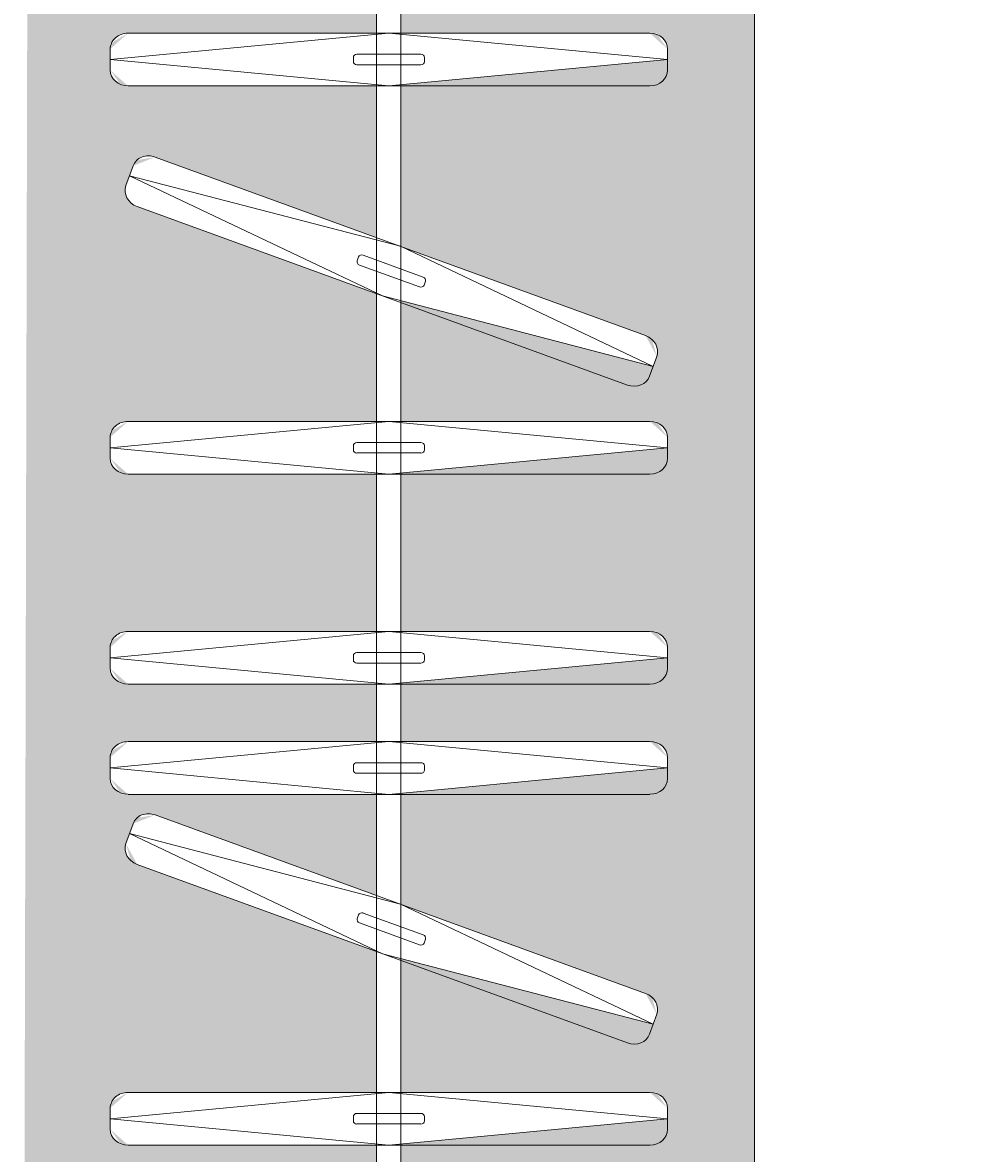
# Model space of a CAD drawing. Units: millimetres. Extents: x 27017497 to 27018854, y 7058029 to 7059154.
# Tile 8 of 91: x 27017623 to 27017651, y 7058166 to 7058200. Entities that reach past the tile are written whole.
import ezdxf

# ---------------------------------------------------------------- set-up
doc = ezdxf.new("R2010")
doc.units = ezdxf.units.MM
for name, color, linetype, lineweight in [('A-ANNO-DIMS', 2, 'Continuous', 18), ('A-FLOR-CASE', 8, 'Continuous', 20), ('A-FLOR-CASE-PATT', 44, 'Continuous', 13)]:
    doc.layers.add(name, color=color, linetype=linetype, lineweight=lineweight)
doc.styles.get("Standard").update_dxf_attribs({"font": 'arial.ttf'})
doc.dimstyles.get("Standard").update_dxf_attribs({"dimtxt": 0.18, "dimasz": 0.18, "dimexe": 0.18, "dimexo": 0.0625, "dimgap": 0.09, "dimtad": 0, "dimtih": 1, "dimtoh": 1, "dimdec": 4, "dimzin": 0, "dimdsep": 46, "dimtxsty": 'Standard', "dimcen": 0.09, "dimadec": 0, "dimazin": 0, "dimtfac": 1, "dimtdec": 4, "dimtofl": 0, "dimtmove": 0, "dimatfit": 3, "dimfxl": 1, "dimtolj": 1, "dimtzin": 0, "dimarcsym": 0})

# ---------------------------------------------------------------- blocks, each defined once
blk = doc.blocks.new('WARDROBE-HANGING')
for p, q in [((0, 21.737), (65.212, 21.737)), ((8.135, 19.153), (7.353, 10.877)), ((8.448, 19.153), (7.822, 19.153)), ((8.135, 19.153), (8.918, 10.877)), ((19.663, 19.153), (18.88, 10.877)), ((19.976, 19.153), (19.35, 19.153)), ((19.663, 19.153), (20.445, 10.877)), ((25.9, 19.153), (25.118, 10.877)), ((26.213, 19.153), (25.587, 19.153)), ((25.9, 19.153), (26.683, 10.877)), ((29.173, 19.153), (28.391, 10.877)), ((29.486, 19.153), (28.86, 19.153)), ((29.173, 19.153), (29.956, 10.877)), ((39.589, 19.153), (38.806, 10.877)), ((39.902, 19.153), (39.276, 19.153)), ((39.589, 19.153), (40.372, 10.877)), ((17.54, 18.619), (16.952, 18.833)), ((37.077, 18.619), (36.488, 18.833)), ((7.353, 18.624), (7.353, 3.13)), ((8.918, 18.624), (8.918, 3.13)), ((16.33, 18.497), (11.031, 3.937)), ((17.246, 18.726), (13.68, 11.217)), ((17.246, 18.726), (15.151, 10.682)), ((18.88, 18.624), (18.88, 3.13)), ((20.445, 18.624), (20.445, 3.13)), ((25.118, 18.624), (25.118, 3.13)), ((26.683, 18.624), (26.683, 3.13)), ((28.391, 18.624), (28.391, 3.13)), ((29.956, 18.624), (29.956, 3.13)), ((35.867, 18.497), (30.567, 3.937)), ((36.783, 18.726), (33.217, 11.217)), ((36.783, 18.726), (34.688, 10.682)), ((38.806, 18.624), (38.806, 3.13)), ((40.372, 18.624), (40.372, 3.13)), ((17.801, 17.962), (12.501, 3.402)), ((37.337, 17.962), (32.038, 3.402)), ((7.979, 11.828), (7.979, 9.927)), ((8.198, 11.934), (8.073, 11.934)), ((8.292, 11.828), (8.292, 9.927)), ((14.594, 11.896), (13.943, 10.11)), ((14.888, 11.789), (14.237, 10.002)), ((14.836, 11.921), (14.718, 11.964)), ((19.506, 11.828), (19.506, 9.927)), ((19.725, 11.934), (19.6, 11.934)), ((19.819, 11.828), (19.819, 9.927)), ((25.744, 11.828), (25.744, 9.927)), ((25.963, 11.934), (25.838, 11.934)), ((26.057, 11.828), (26.057, 9.927)), ((29.017, 11.828), (29.017, 9.927)), ((29.236, 11.934), (29.111, 11.934)), ((29.33, 11.828), (29.33, 9.927)), ((34.13, 11.896), (33.48, 10.11)), ((34.425, 11.789), (33.774, 10.002)), ((34.372, 11.921), (34.255, 11.964)), ((39.432, 11.828), (39.432, 9.927)), ((39.652, 11.934), (39.526, 11.934)), ((39.745, 11.828), (39.745, 9.927)), ((0, 11.231), (65.212, 11.231)), ((11.585, 3.173), (13.68, 11.217)), ((31.122, 3.173), (33.217, 11.217)), ((8.135, 2.602), (7.353, 10.877)), ((8.135, 2.602), (8.918, 10.877)), ((19.663, 2.602), (18.88, 10.877)), ((19.663, 2.602), (20.445, 10.877)), ((25.9, 2.602), (25.118, 10.877)), ((25.9, 2.602), (26.683, 10.877)), ((29.173, 2.602), (28.391, 10.877)), ((29.173, 2.602), (29.956, 10.877)), ((39.589, 2.602), (38.806, 10.877)), ((39.589, 2.602), (40.372, 10.877)), ((0, 10.506), (65.212, 10.506)), ((11.585, 3.173), (15.151, 10.682)), ((31.122, 3.173), (34.688, 10.682)), ((8.198, 9.821), (8.073, 9.821)), ((14.113, 9.935), (13.995, 9.978)), ((19.725, 9.821), (19.6, 9.821)), ((25.963, 9.821), (25.838, 9.821)), ((29.236, 9.821), (29.111, 9.821)), ((33.65, 9.935), (33.532, 9.978)), ((39.652, 9.821), (39.526, 9.821)), ((11.879, 3.066), (11.291, 3.28)), ((31.416, 3.066), (30.828, 3.28)), ((8.448, 2.602), (7.822, 2.602)), ((19.976, 2.602), (19.35, 2.602)), ((26.213, 2.602), (25.587, 2.602)), ((29.486, 2.602), (28.86, 2.602)), ((39.902, 2.602), (39.276, 2.602))]:
    blk.add_line(p, q)
for centre, major_axis, start_param, end_param in [((7.822, 18.624), (0, 0.528), 0, 1.570796), ((8.448, 18.624), (0, 0.528), 4.712389, 6.283185), ((19.35, 18.624), (0, 0.528), 0, 1.570796), ((19.976, 18.624), (0, 0.528), 4.712389, 6.283185), ((25.587, 18.624), (0, 0.528), 0, 1.570796), ((26.213, 18.624), (0, 0.528), 4.712389, 6.283185), ((28.86, 18.624), (0, 0.528), 0, 1.570796), ((29.486, 18.624), (0, 0.528), 4.712389, 6.283185), ((39.276, 18.624), (0, 0.528), 0, 1.570796), ((39.902, 18.624), (0, 0.528), 4.712389, 6.283185), ((16.771, 18.336), (0.181, 0.496), 0, 1.570796), ((36.308, 18.336), (0.181, 0.496), 0, 1.570796), ((17.359, 18.122), (0.181, 0.496), -1.570796, 0), ((36.896, 18.122), (0.181, 0.496), -1.570796, 0), ((8.073, 11.828), (0, 0.106), 0, 1.570796), ((8.198, 11.828), (0, 0.106), -1.570796, 0), ((14.682, 11.864), (0.0361, 0.0993), 0, 1.570796), ((14.8, 11.821), (0.0361, 0.0993), 4.712389, 6.283185), ((19.6, 11.828), (0, 0.106), 0, 1.570796), ((19.725, 11.828), (0, 0.106), -1.570796, 0), ((25.838, 11.828), (0, 0.106), 0, 1.570796), ((25.963, 11.828), (0, 0.106), -1.570796, 0), ((29.111, 11.828), (0, 0.106), 0, 1.570796), ((29.236, 11.828), (0, 0.106), -1.570796, 0), ((34.219, 11.864), (0.0361, 0.0993), 0, 1.570796), ((34.336, 11.821), (0.0361, 0.0993), 4.712389, 6.283185), ((39.526, 11.828), (0, 0.106), 0, 1.570796), ((39.652, 11.828), (0, 0.106), -1.570796, 0), ((14.032, 10.077), (0.0361, 0.0993), 1.570796, 3.141593), ((33.568, 10.077), (0.0361, 0.0993), 1.570796, 3.141593), ((8.073, 9.927), (0, 0.106), 1.570796, 3.141593), ((8.198, 9.927), (0, 0.106), 3.141593, 4.712389), ((14.149, 10.035), (0.0361, 0.0993), 3.141593, 4.712389), ((19.6, 9.927), (0, 0.106), 1.570796, 3.141593), ((19.725, 9.927), (0, 0.106), 3.141593, 4.712389), ((25.838, 9.927), (0, 0.106), 1.570796, 3.141593), ((25.963, 9.927), (0, 0.106), 3.141593, 4.712389), ((29.111, 9.927), (0, 0.106), 1.570796, 3.141593), ((29.236, 9.927), (0, 0.106), 3.141593, 4.712389), ((33.686, 10.035), (0.0361, 0.0993), 3.141593, 4.712389), ((39.526, 9.927), (0, 0.106), 1.570796, 3.141593), ((39.652, 9.927), (0, 0.106), 3.141593, 4.712389), ((11.472, 3.777), (0.181, 0.496), 1.570796, 3.141593), ((31.008, 3.777), (0.181, 0.496), 1.570796, 3.141593), ((12.06, 3.562), (0.181, 0.496), 3.141593, 4.712389), ((31.597, 3.562), (0.181, 0.496), 3.141593, 4.712389), ((7.822, 3.13), (0, 0.528), 1.570796, 3.141593), ((8.448, 3.13), (0, 0.528), 3.141593, 4.712389), ((19.35, 3.13), (0, 0.528), 1.570796, 3.141593), ((19.976, 3.13), (0, 0.528), 3.141593, 4.712389), ((25.587, 3.13), (0, 0.528), 1.570796, 3.141593), ((26.213, 3.13), (0, 0.528), 3.141593, 4.712389), ((28.86, 3.13), (0, 0.528), 1.570796, 3.141593), ((29.486, 3.13), (0, 0.528), 3.141593, 4.712389), ((39.276, 3.13), (0, 0.528), 1.570796, 3.141593), ((39.902, 3.13), (0, 0.528), 3.141593, 4.712389)]:
    blk.add_ellipse(centre, major_axis=major_axis, ratio=0.888892, start_param=start_param, end_param=end_param)
blk = doc.blocks.new('*D47')
at = {"layer": 'A-ANNO-DIMS', "color": 0, "lineweight": -2, "transparency": 16777216}
for p, q in [((27017561.166, 7058294.35), (27017561.166, 7058028.6)), ((27018790.606, 7058294.35), (27018790.606, 7058028.6)), ((27017561.346, 7058028.78), (27018175.431, 7058028.78)), ((27018790.426, 7058028.78), (27018176.341, 7058028.78))]:
    blk.add_line(p, q, dxfattribs=at)
at = {"layer": 'A-ANNO-DIMS', "color": 0, "transparency": 16777216}
for points in [[(27017561.346, 7058028.81), (27017561.346, 7058028.75), (27017561.166, 7058028.78)], [(27018790.426, 7058028.81), (27018790.426, 7058028.75), (27018790.606, 7058028.78)]]:
    blk.add_solid(points, dxfattribs=at)
at = {"layer": 'Defpoints', "color": 0, "transparency": 16777216}
for p in [(27017561.166, 7058294.412), (27018790.606, 7058294.412), (27018790.606, 7058028.78)]:
    blk.add_point(p, dxfattribs=at)
at = {"layer": 'A-ANNO-DIMS', "color": 0, "transparency": 16777216, "insert": (27018175.886, 7058028.78), "char_height": 0.18, "attachment_point": 5}
blk.add_mtext('\\A1;1229.4', dxfattribs=at)
blk = doc.blocks.new('*D48')
at = {"layer": 'A-ANNO-DIMS', "color": 0, "lineweight": -2, "transparency": 16777216}
for p, q in [((27018463.498, 7058622.912), (27017497.536, 7058622.912)), ((27017497.716, 7058622.732), (27017497.716, 7058357.753)), ((27017497.716, 7058092.41), (27017497.716, 7058357.389)), ((27018555.129, 7058092.23), (27017497.536, 7058092.23))]:
    blk.add_line(p, q, dxfattribs=at)
at = {"layer": 'A-ANNO-DIMS', "color": 0, "transparency": 16777216}
for points in [[(27017497.686, 7058622.732), (27017497.746, 7058622.732), (27017497.716, 7058622.912)], [(27017497.686, 7058092.41), (27017497.746, 7058092.41), (27017497.716, 7058092.23)]]:
    blk.add_solid(points, dxfattribs=at)
at = {"layer": 'Defpoints', "color": 0, "transparency": 16777216}
for p in [(27018463.561, 7058622.912), (27017497.716, 7058092.23), (27018555.192, 7058092.23)]:
    blk.add_point(p, dxfattribs=at)
at = {"layer": 'A-ANNO-DIMS', "color": 0, "transparency": 16777216, "insert": (27017497.716, 7058357.571), "char_height": 0.18, "attachment_point": 5}
blk.add_mtext('\\A1;530.7', dxfattribs=at)

msp = doc.modelspace()

# ---------------------------------------------------------------- hatches: boundary and pattern name
at = {"layer": 'A-FLOR-CASE-PATT'}
h = msp.add_hatch(color=256, dxfattribs=at)
h.dxf.hatch_style = 1
edge = h.paths.add_edge_path()
edge.add_line((27017644.461, 7058207.1), (27017639.716, 7058207.1))
edge.add_line((27017639.716, 7058207.1), (27017639.716, 7058207.055))
edge.add_line((27017639.716, 7058207.055), (27017633.955, 7058207.055))
edge.add_line((27017633.955, 7058207.055), (27017633.955, 7058203.02))
edge.add_line((27017633.955, 7058203.02), (27017641.542, 7058203.02))
edge.add_ellipse((27017641.349, 7058202.551), major_axis=(0.528, 0), ratio=0.888892, start_angle=0, end_angle=90, ccw=False)
edge.add_line((27017641.877, 7058202.551), (27017641.877, 7058202.238))
edge.add_line((27017641.877, 7058202.238), (27017633.955, 7058201.488))
edge.add_line((27017633.955, 7058201.488), (27017633.955, 7058199.747))
edge.add_line((27017633.955, 7058199.747), (27017641.542, 7058199.747))
edge.add_ellipse((27017641.349, 7058199.277), major_axis=(0.528, 0), ratio=0.888892, start_angle=0, end_angle=90, ccw=False)
edge.add_line((27017641.877, 7058199.277), (27017641.877, 7058198.964))
edge.add_line((27017641.877, 7058198.964), (27017633.955, 7058198.215))
edge.add_line((27017633.955, 7058198.215), (27017633.955, 7058193.415))
edge.add_line((27017633.955, 7058193.415), (27017641.403, 7058190.704))
edge.add_ellipse((27017641.06, 7058190.329), major_axis=(0.496, -0.181), ratio=0.888892, start_angle=0, end_angle=90, ccw=False)
edge.add_line((27017641.557, 7058190.148), (27017641.45, 7058189.854))
edge.add_line((27017641.45, 7058189.854), (27017633.955, 7058191.806))
edge.add_line((27017633.955, 7058191.806), (27017633.955, 7058188.22))
edge.add_line((27017633.955, 7058188.22), (27017641.542, 7058188.22))
edge.add_ellipse((27017641.349, 7058187.75), major_axis=(0.528, 0), ratio=0.888892, start_angle=0, end_angle=90, ccw=False)
edge.add_line((27017641.877, 7058187.75), (27017641.877, 7058187.437))
edge.add_line((27017641.877, 7058187.437), (27017633.955, 7058186.688))
edge.add_line((27017633.955, 7058186.688), (27017633.955, 7058181.982))
edge.add_line((27017633.955, 7058181.982), (27017641.542, 7058181.982))
edge.add_ellipse((27017641.349, 7058181.513), major_axis=(0.528, 0), ratio=0.888892, start_angle=0, end_angle=90, ccw=False)
edge.add_line((27017641.877, 7058181.513), (27017641.877, 7058181.199))
edge.add_line((27017641.877, 7058181.199), (27017633.955, 7058180.45))
edge.add_line((27017633.955, 7058180.45), (27017633.955, 7058178.709))
edge.add_line((27017633.955, 7058178.709), (27017641.542, 7058178.709))
edge.add_ellipse((27017641.349, 7058178.239), major_axis=(0.528, 0), ratio=0.888892, start_angle=0, end_angle=90, ccw=False)
edge.add_line((27017641.877, 7058178.239), (27017641.877, 7058177.926))
edge.add_line((27017641.877, 7058177.926), (27017633.955, 7058177.177))
edge.add_line((27017633.955, 7058177.177), (27017633.955, 7058173.878))
edge.add_line((27017633.955, 7058173.878), (27017641.403, 7058171.167))
edge.add_ellipse((27017641.06, 7058170.792), major_axis=(0.496, -0.181), ratio=0.888892, start_angle=0, end_angle=90, ccw=False)
edge.add_line((27017641.557, 7058170.611), (27017641.45, 7058170.317))
edge.add_line((27017641.45, 7058170.317), (27017633.955, 7058172.269))
edge.add_line((27017633.955, 7058172.269), (27017633.955, 7058168.293))
edge.add_line((27017633.955, 7058168.293), (27017641.542, 7058168.293))
edge.add_ellipse((27017641.349, 7058167.824), major_axis=(0.528, 0), ratio=0.888892, start_angle=0, end_angle=90, ccw=False)
edge.add_line((27017641.877, 7058167.824), (27017641.877, 7058167.511))
edge.add_line((27017641.877, 7058167.511), (27017633.955, 7058166.762))
edge.add_line((27017633.955, 7058166.762), (27017633.955, 7058160.389))
edge.add_line((27017633.955, 7058160.389), (27017641.542, 7058160.389))
edge.add_ellipse((27017641.349, 7058159.92), major_axis=(0.528, 0), ratio=0.888892, start_angle=0, end_angle=90, ccw=False)
edge.add_line((27017641.877, 7058159.92), (27017641.877, 7058159.607))
edge.add_line((27017641.877, 7058159.607), (27017633.955, 7058158.858))
edge.add_line((27017633.955, 7058158.858), (27017633.955, 7058157.116))
edge.add_line((27017633.955, 7058157.116), (27017641.542, 7058157.116))
edge.add_ellipse((27017641.349, 7058156.647), major_axis=(0.528, 0), ratio=0.888892, start_angle=0, end_angle=90, ccw=False)
edge.add_line((27017641.877, 7058156.647), (27017641.877, 7058156.334))
edge.add_line((27017641.877, 7058156.334), (27017633.955, 7058155.585))
edge.add_line((27017633.955, 7058155.585), (27017633.955, 7058150.784))
edge.add_line((27017633.955, 7058150.784), (27017641.403, 7058148.073))
edge.add_ellipse((27017641.06, 7058147.698), major_axis=(0.496, -0.181), ratio=0.888892, start_angle=0, end_angle=90, ccw=False)
edge.add_line((27017641.557, 7058147.517), (27017641.45, 7058147.223))
edge.add_line((27017641.45, 7058147.223), (27017633.955, 7058149.175))
edge.add_line((27017633.955, 7058149.175), (27017633.955, 7058145.589))
edge.add_line((27017633.955, 7058145.589), (27017641.542, 7058145.589))
edge.add_ellipse((27017641.349, 7058145.119), major_axis=(0.528, 0), ratio=0.888892, start_angle=0, end_angle=90, ccw=False)
edge.add_line((27017641.877, 7058145.119), (27017641.877, 7058144.806))
edge.add_line((27017641.877, 7058144.806), (27017633.955, 7058144.057))
edge.add_line((27017633.955, 7058144.057), (27017633.955, 7058141.912))
edge.add_line((27017633.955, 7058141.912), (27017644.461, 7058141.912))
edge.add_line((27017644.461, 7058141.912), (27017644.461, 7058207.1))
edge = h.paths.add_edge_path()
edge.add_ellipse((27017626.287, 7058195.04), major_axis=(0.496, -0.181), ratio=0.888892, start_angle=180, end_angle=270, ccw=False)
edge.add_line((27017625.79, 7058195.22), (27017626.063, 7058195.97))
edge.add_ellipse((27017626.501, 7058195.628), major_axis=(0.496, -0.181), ratio=0.888892, start_angle=90, end_angle=180, ccw=False)
edge.add_line((27017626.661, 7058196.069), (27017633.23, 7058193.678))
edge.add_line((27017633.23, 7058193.678), (27017633.23, 7058198.182))
edge.add_line((27017633.23, 7058198.182), (27017625.661, 7058198.182))
edge.add_ellipse((27017625.854, 7058198.651), major_axis=(0.528, 0), ratio=0.888892, start_angle=180, end_angle=270, ccw=False)
edge.add_line((27017625.326, 7058198.651), (27017625.326, 7058199.449))
edge.add_ellipse((27017625.854, 7058199.277), major_axis=(0.528, 0), ratio=0.888892, start_angle=90, end_angle=180, ccw=False)
edge.add_line((27017625.854, 7058199.747), (27017633.23, 7058199.747))
edge.add_line((27017633.23, 7058199.747), (27017633.23, 7058201.455))
edge.add_line((27017633.23, 7058201.455), (27017625.661, 7058201.455))
edge.add_ellipse((27017625.854, 7058201.924), major_axis=(0.528, 0), ratio=0.888892, start_angle=180, end_angle=270, ccw=False)
edge.add_line((27017625.326, 7058201.924), (27017625.326, 7058202.722))
edge.add_ellipse((27017625.854, 7058202.551), major_axis=(0.528, 0), ratio=0.888892, start_angle=90, end_angle=180, ccw=False)
edge.add_line((27017625.854, 7058203.02), (27017633.23, 7058203.02))
edge.add_line((27017633.23, 7058203.02), (27017633.23, 7058207.055))
edge.add_line((27017633.23, 7058207.055), (27017622.865, 7058207.055))
edge.add_line((27017622.865, 7058207.055), (27017622.865, 7058201.7))
edge.add_line((27017622.865, 7058201.7), (27017622.724, 7058141.912))
edge.add_line((27017622.724, 7058141.912), (27017633.23, 7058141.912))
edge.add_line((27017633.23, 7058141.912), (27017633.23, 7058144.024))
edge.add_line((27017633.23, 7058144.024), (27017625.661, 7058144.024))
edge.add_ellipse((27017625.854, 7058144.493), major_axis=(0.528, 0), ratio=0.888892, start_angle=180, end_angle=270, ccw=False)
edge.add_line((27017625.326, 7058144.493), (27017625.326, 7058145.291))
edge.add_ellipse((27017625.854, 7058145.119), major_axis=(0.528, 0), ratio=0.888892, start_angle=90, end_angle=180, ccw=False)
edge.add_line((27017625.854, 7058145.589), (27017633.23, 7058145.589))
edge.add_line((27017633.23, 7058145.589), (27017633.23, 7058149.382))
edge.add_line((27017633.23, 7058149.382), (27017625.944, 7058152.034))
edge.add_ellipse((27017626.287, 7058152.409), major_axis=(0.496, -0.181), ratio=0.888892, start_angle=180, end_angle=270, ccw=False)
edge.add_line((27017625.79, 7058152.59), (27017626.063, 7058153.34))
edge.add_ellipse((27017626.501, 7058152.997), major_axis=(0.496, -0.181), ratio=0.888892, start_angle=90, end_angle=180, ccw=False)
edge.add_line((27017626.661, 7058153.439), (27017633.23, 7058151.048))
edge.add_line((27017633.23, 7058151.048), (27017633.23, 7058155.551))
edge.add_line((27017633.23, 7058155.551), (27017625.661, 7058155.551))
edge.add_ellipse((27017625.854, 7058156.021), major_axis=(0.528, 0), ratio=0.888892, start_angle=180, end_angle=270, ccw=False)
edge.add_line((27017625.326, 7058156.021), (27017625.326, 7058156.819))
edge.add_ellipse((27017625.854, 7058156.647), major_axis=(0.528, 0), ratio=0.888892, start_angle=90, end_angle=180, ccw=False)
edge.add_line((27017625.854, 7058157.116), (27017633.23, 7058157.116))
edge.add_line((27017633.23, 7058157.116), (27017633.23, 7058158.824))
edge.add_line((27017633.23, 7058158.824), (27017625.661, 7058158.824))
edge.add_ellipse((27017625.854, 7058159.294), major_axis=(0.528, 0), ratio=0.888892, start_angle=180, end_angle=270, ccw=False)
edge.add_line((27017625.326, 7058159.294), (27017625.326, 7058160.092))
edge.add_ellipse((27017625.854, 7058159.92), major_axis=(0.528, 0), ratio=0.888892, start_angle=90, end_angle=180, ccw=False)
edge.add_line((27017625.854, 7058160.389), (27017633.23, 7058160.389))
edge.add_line((27017633.23, 7058160.389), (27017633.23, 7058166.728))
edge.add_line((27017633.23, 7058166.728), (27017625.661, 7058166.728))
edge.add_ellipse((27017625.854, 7058167.198), major_axis=(0.528, 0), ratio=0.888892, start_angle=180, end_angle=270, ccw=False)
edge.add_line((27017625.326, 7058167.198), (27017625.326, 7058167.996))
edge.add_ellipse((27017625.854, 7058167.824), major_axis=(0.528, 0), ratio=0.888892, start_angle=90, end_angle=180, ccw=False)
edge.add_line((27017625.854, 7058168.293), (27017633.23, 7058168.293))
edge.add_line((27017633.23, 7058168.293), (27017633.23, 7058172.476))
edge.add_line((27017633.23, 7058172.476), (27017625.944, 7058175.128))
edge.add_ellipse((27017626.287, 7058175.503), major_axis=(0.496, -0.181), ratio=0.888892, start_angle=180, end_angle=270, ccw=False)
edge.add_line((27017625.79, 7058175.684), (27017626.063, 7058176.433))
edge.add_ellipse((27017626.501, 7058176.091), major_axis=(0.496, -0.181), ratio=0.888892, start_angle=90, end_angle=180, ccw=False)
edge.add_line((27017626.661, 7058176.533), (27017633.23, 7058174.142))
edge.add_line((27017633.23, 7058174.142), (27017633.23, 7058177.144))
edge.add_line((27017633.23, 7058177.144), (27017625.661, 7058177.144))
edge.add_ellipse((27017625.854, 7058177.613), major_axis=(0.528, 0), ratio=0.888892, start_angle=180, end_angle=270, ccw=False)
edge.add_line((27017625.326, 7058177.613), (27017625.326, 7058178.411))
edge.add_ellipse((27017625.854, 7058178.239), major_axis=(0.528, 0), ratio=0.888892, start_angle=90, end_angle=180, ccw=False)
edge.add_line((27017625.854, 7058178.709), (27017633.23, 7058178.709))
edge.add_line((27017633.23, 7058178.709), (27017633.23, 7058180.417))
edge.add_line((27017633.23, 7058180.417), (27017625.661, 7058180.417))
edge.add_ellipse((27017625.854, 7058180.886), major_axis=(0.528, 0), ratio=0.888892, start_angle=180, end_angle=270, ccw=False)
edge.add_line((27017625.326, 7058180.886), (27017625.326, 7058181.684))
edge.add_ellipse((27017625.854, 7058181.513), major_axis=(0.528, 0), ratio=0.888892, start_angle=90, end_angle=180, ccw=False)
edge.add_line((27017625.854, 7058181.982), (27017633.23, 7058181.982))
edge.add_line((27017633.23, 7058181.982), (27017633.23, 7058186.655))
edge.add_line((27017633.23, 7058186.655), (27017625.661, 7058186.655))
edge.add_ellipse((27017625.854, 7058187.124), major_axis=(0.528, 0), ratio=0.888892, start_angle=180, end_angle=270, ccw=False)
edge.add_line((27017625.326, 7058187.124), (27017625.326, 7058187.922))
edge.add_ellipse((27017625.854, 7058187.75), major_axis=(0.528, 0), ratio=0.888892, start_angle=90, end_angle=180, ccw=False)
edge.add_line((27017625.854, 7058188.22), (27017633.23, 7058188.22))
edge.add_line((27017633.23, 7058188.22), (27017633.23, 7058192.013))
edge.add_line((27017633.23, 7058192.013), (27017625.944, 7058194.665))

# ---------------------------------------------------------------- block references
at = {"layer": 'A-FLOR-CASE', "rotation": 270}
msp.add_blockref('WARDROBE-HANGING', (27017622.724, 7058207.1), dxfattribs=at)

# ---------------------------------------------------------------- dimensions: what is measured, and where the dimension line sits
at = {"layer": 'A-ANNO-DIMS'}
dim = msp.add_linear_dim(base=(27017497.716, 7058092.23), p1=(27018463.561, 7058622.912), p2=(27018555.192, 7058092.23), angle=90, dimstyle='Standard', override={"dimdec": 1, "dimlfac": 1, "dimrnd": 0, "dimzin": 0, "dimdsep": 46, "dimlunit": 2}, dxfattribs=at)
dim.commit()
dim.dimension.update_dxf_attribs({"geometry": '*D48', "text_midpoint": (27017497.716, 7058357.571)})
dim = msp.add_linear_dim(base=(27018790.606, 7058028.78), p1=(27017561.166, 7058294.412), p2=(27018790.606, 7058294.412), dimstyle='Standard', override={"dimdec": 1, "dimlfac": 1, "dimrnd": 0, "dimzin": 0, "dimdsep": 46, "dimlunit": 2}, dxfattribs=at)
dim.commit()
dim.dimension.update_dxf_attribs({"geometry": '*D47', "text_midpoint": (27018175.886, 7058028.78)})

doc.saveas('drawing.dxf')
